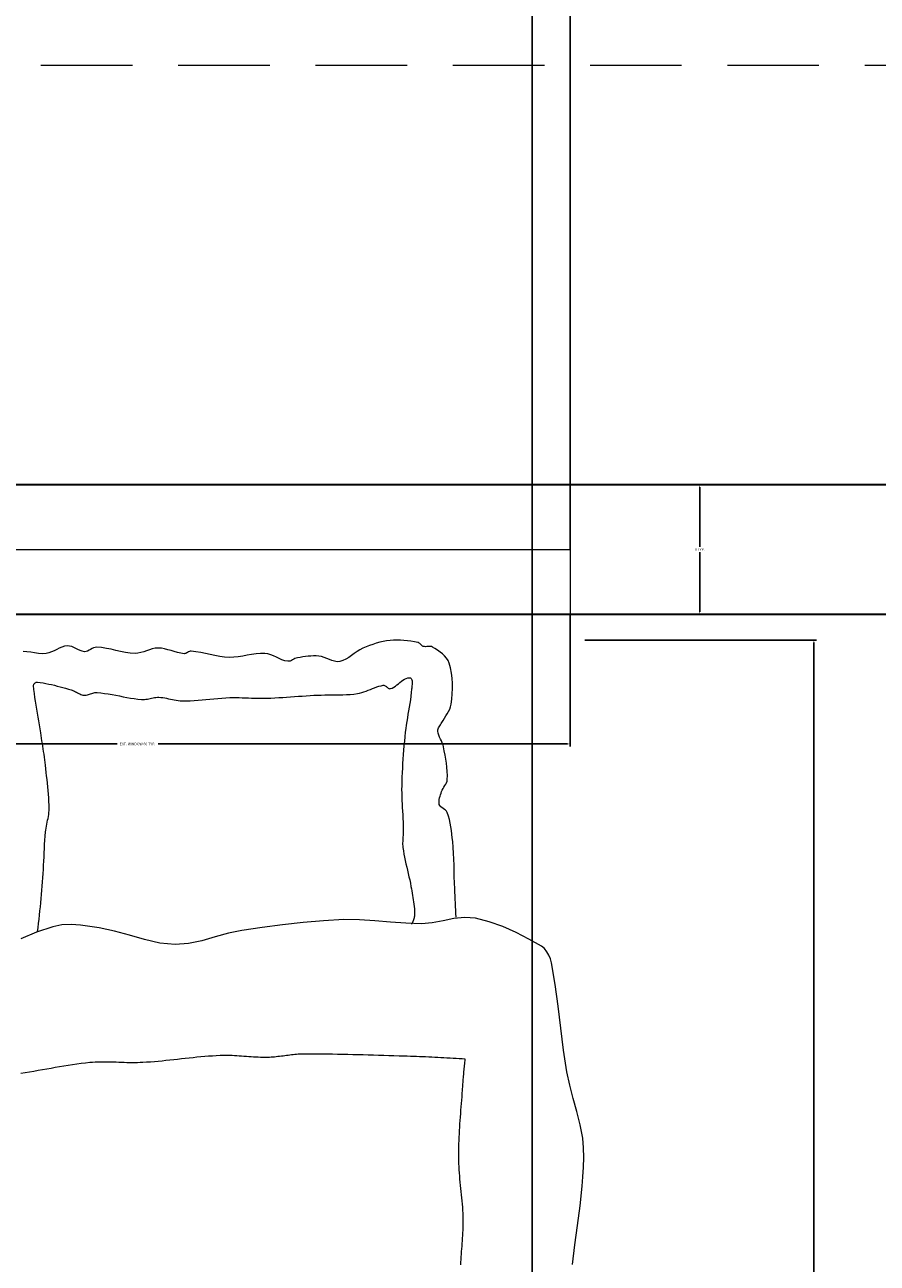
# Model space of a CAD drawing. Units: inches. Extents: x 1770 to 2988, y 1161 to 3221.
# Tile 18 of 44: x 2229 to 2289, y 2323 to 2409. Entities that reach past the tile are written whole.
import ezdxf

# ---------------------------------------------------------------- set-up
doc = ezdxf.new("R2010")
doc.units = ezdxf.units.IN
doc.linetypes.add('DASHED2', pattern=[9.525, 6.35, -3.175])
for name, color, linetype, lineweight in [('A-ANNO-DIMS', 2, 'Continuous', 18), ('A-FURN', 8, 'Continuous', 13), ('A-GLAZ', 4, 'Continuous', 18), ('A-ROOF-OVHD', 7, 'DASHED2', 18), ('A-WALL', 7, 'Continuous', 35)]:
    doc.layers.add(name, color=color, linetype=linetype, lineweight=lineweight)
doc.styles.get("Standard").update_dxf_attribs({"font": 'arial.ttf'})
doc.dimstyles.get("Standard").update_dxf_attribs({"dimtxt": 0.18, "dimasz": 0.18, "dimexe": 0.18, "dimexo": 0.0625, "dimgap": 0.09, "dimtad": 0, "dimtih": 1, "dimtoh": 1, "dimdec": 4, "dimzin": 0, "dimdsep": 46, "dimtxsty": 'Standard', "dimcen": 0.09, "dimadec": 0, "dimazin": 0, "dimtfac": 1, "dimtdec": 4, "dimtofl": 0, "dimtmove": 0, "dimatfit": 3, "dimfxl": 1, "dimtolj": 1, "dimtzin": 0, "dimarcsym": 0})

# ---------------------------------------------------------------- blocks, each defined once
blk = doc.blocks.new('BED-DOUBLE-PLAN')
for p, q in [((38.413, 105.766), (38.234, 105.676)), ((38.593, 105.854), (38.413, 105.766)), ((38.774, 105.931), (38.593, 105.854)), ((38.959, 105.987), (38.774, 105.931)), ((39.151, 106.014), (38.959, 105.987)), ((39.305, 106.003), (39.151, 106.014)), ((39.454, 105.962), (39.305, 106.003)), ((39.599, 105.9), (39.454, 105.962)), ((39.744, 105.827), (39.599, 105.9)), ((39.888, 105.751), (39.744, 105.827)), ((40.034, 105.684), (39.888, 105.751)), ((40.766, 105.763), (40.662, 105.704)), ((40.87, 105.822), (40.766, 105.763)), ((40.976, 105.874), (40.87, 105.822)), ((41.084, 105.909), (40.976, 105.874)), ((41.195, 105.919), (41.084, 105.909)), ((41.529, 105.893), (41.195, 105.919)), ((41.861, 105.841), (41.529, 105.893)), ((42.191, 105.773), (41.861, 105.841)), ((42.521, 105.698), (42.191, 105.773)), ((45.042, 105.801), (44.844, 105.741)), ((45.243, 105.843), (45.042, 105.801)), ((45.446, 105.858), (45.243, 105.843)), ((45.675, 105.843), (45.446, 105.858)), ((45.901, 105.804), (45.675, 105.843)), ((46.126, 105.748), (45.901, 105.804)), ((46.349, 105.683), (46.126, 105.748)), ((59.45, 105.749), (59.252, 105.623)), ((59.658, 105.853), (59.45, 105.749)), ((59.885, 105.946), (59.658, 105.853)), ((60.115, 106.035), (59.885, 105.946)), ((60.348, 106.118), (60.115, 106.035)), ((60.582, 106.193), (60.348, 106.118)), ((60.819, 106.26), (60.582, 106.193)), ((61.059, 106.316), (60.819, 106.26)), ((61.3, 106.362), (61.059, 106.316)), ((61.543, 106.394), (61.3, 106.362)), ((61.783, 106.412), (61.543, 106.394)), ((62.023, 106.417), (61.783, 106.412)), ((62.265, 106.41), (62.023, 106.417)), ((62.506, 106.393), (62.265, 106.41)), ((62.747, 106.368), (62.506, 106.393)), ((62.987, 106.335), (62.747, 106.368)), ((63.226, 106.297), (62.987, 106.335)), ((63.464, 106.255), (63.226, 106.297)), ((63.519, 106.237), (63.464, 106.255)), ((63.567, 106.207), (63.519, 106.237)), ((63.612, 106.167), (63.567, 106.207)), ((63.655, 106.123), (63.612, 106.167)), ((63.698, 106.078), (63.655, 106.123)), ((63.742, 106.036), (63.698, 106.078)), ((63.79, 106), (63.742, 106.036)), ((63.842, 105.976), (63.79, 106)), ((63.921, 105.96), (63.842, 105.976)), ((64.003, 105.957), (63.921, 105.96)), ((64.087, 105.963), (64.003, 105.957)), ((64.171, 105.972), (64.087, 105.963)), ((64.255, 105.978), (64.171, 105.972)), ((64.335, 105.976), (64.255, 105.978)), ((64.412, 105.962), (64.335, 105.976)), ((64.483, 105.93), (64.412, 105.962)), ((64.655, 105.82), (64.483, 105.93)), ((64.831, 105.707), (64.655, 105.82)), ((36.348, 105.604), (36.086, 105.618)), ((36.614, 105.569), (36.348, 105.604)), ((36.882, 105.525), (36.614, 105.569)), ((37.15, 105.487), (36.882, 105.525)), ((37.417, 105.469), (37.15, 105.487)), ((37.679, 105.483), (37.417, 105.469)), ((37.869, 105.525), (37.679, 105.483)), ((38.054, 105.593), (37.869, 105.525)), ((38.234, 105.676), (38.054, 105.593)), ((40.183, 105.634), (40.034, 105.684)), ((40.337, 105.61), (40.183, 105.634)), ((40.448, 105.619), (40.337, 105.61)), ((40.556, 105.654), (40.448, 105.619)), ((40.662, 105.704), (40.556, 105.654)), ((42.85, 105.623), (42.521, 105.698)), ((43.18, 105.557), (42.85, 105.623)), ((43.512, 105.51), (43.18, 105.557)), ((43.846, 105.489), (43.512, 105.51)), ((44.05, 105.503), (43.846, 105.489)), ((44.25, 105.544), (44.05, 105.503)), ((44.449, 105.603), (44.25, 105.544)), ((44.646, 105.672), (44.449, 105.603)), ((44.844, 105.741), (44.646, 105.672)), ((46.572, 105.616), (46.349, 105.683)), ((46.796, 105.553), (46.572, 105.616)), ((47.022, 105.502), (46.796, 105.553)), ((47.25, 105.469), (47.022, 105.502)), ((47.314, 105.472), (47.25, 105.469)), ((47.375, 105.492), (47.314, 105.472)), ((47.436, 105.521), (47.375, 105.492)), ((47.495, 105.556), (47.436, 105.521)), ((47.555, 105.592), (47.495, 105.556)), ((47.615, 105.622), (47.555, 105.592)), ((47.677, 105.641), (47.615, 105.622)), ((47.741, 105.646), (47.677, 105.641)), ((48.074, 105.608), (47.741, 105.646)), ((48.406, 105.552), (48.074, 105.608)), ((48.736, 105.485), (48.406, 105.552)), ((49.065, 105.414), (48.736, 105.485)), ((49.395, 105.345), (49.065, 105.414)), ((49.725, 105.284), (49.395, 105.345)), ((50.057, 105.239), (49.725, 105.284)), ((50.391, 105.215), (50.057, 105.239)), ((50.701, 105.221), (50.391, 105.215)), ((51.01, 105.253), (50.701, 105.221)), ((51.318, 105.302), (51.01, 105.253)), ((51.626, 105.359), (51.318, 105.302)), ((51.934, 105.415), (51.626, 105.359)), ((52.242, 105.46), (51.934, 105.415)), ((52.551, 105.485), (52.242, 105.46)), ((52.86, 105.482), (52.551, 105.485)), ((53.065, 105.451), (52.86, 105.482)), ((53.264, 105.392), (53.065, 105.451)), ((53.459, 105.314), (53.264, 105.392)), ((53.652, 105.225), (53.459, 105.314)), ((53.845, 105.135), (53.652, 105.225)), ((54.039, 105.052), (53.845, 105.135)), ((54.237, 104.985), (54.039, 105.052)), ((54.441, 104.943), (54.237, 104.985)), ((54.528, 104.942), (54.441, 104.943)), ((54.613, 104.962), (54.528, 104.942)), ((54.696, 104.995), (54.613, 104.962)), ((54.779, 105.038), (54.696, 104.995)), ((54.861, 105.083), (54.779, 105.038)), ((54.944, 105.127), (54.861, 105.083)), ((55.029, 105.163), (54.944, 105.127)), ((55.116, 105.186), (55.029, 105.163)), ((55.3, 105.216), (55.116, 105.186)), ((55.484, 105.245), (55.3, 105.216)), ((55.669, 105.271), (55.484, 105.245)), ((55.855, 105.292), (55.669, 105.271)), ((56.041, 105.308), (55.855, 105.292)), ((56.227, 105.316), (56.041, 105.308)), ((56.413, 105.315), (56.227, 105.316)), ((56.598, 105.304), (56.413, 105.315)), ((56.783, 105.272), (56.598, 105.304)), ((56.966, 105.215), (56.783, 105.272)), ((57.147, 105.142), (56.966, 105.215)), ((57.327, 105.066), (57.147, 105.142)), ((57.506, 104.996), (57.327, 105.066)), ((57.686, 104.943), (57.506, 104.996)), ((57.868, 104.916), (57.686, 104.943)), ((58.051, 104.927), (57.868, 104.916)), ((58.271, 104.989), (58.051, 104.927)), ((58.479, 105.084), (58.271, 104.989)), ((58.677, 105.205), (58.479, 105.084)), ((58.869, 105.341), (58.677, 105.205)), ((59.06, 105.484), (58.869, 105.341)), ((59.252, 105.623), (59.06, 105.484)), ((65.005, 105.587), (64.831, 105.707)), ((65.17, 105.459), (65.005, 105.587)), ((65.323, 105.321), (65.17, 105.459)), ((65.456, 105.17), (65.323, 105.321)), ((65.565, 105.005), (65.456, 105.17)), ((65.644, 104.823), (65.565, 105.005)), ((65.74, 104.478), (65.644, 104.823)), ((65.806, 104.126), (65.74, 104.478)), ((65.847, 103.768), (65.806, 104.126)), ((36.815, 103.265), (36.816, 103.295)), ((36.837, 102.989), (36.815, 103.265)), ((36.816, 103.295), (36.824, 103.324)), ((36.824, 103.324), (36.836, 103.353)), ((36.836, 103.353), (36.854, 103.381)), ((36.854, 103.381), (36.875, 103.407)), ((36.875, 103.407), (36.9, 103.431)), ((36.9, 103.431), (36.927, 103.452)), ((36.927, 103.452), (36.956, 103.47)), ((36.956, 103.47), (36.986, 103.485)), ((36.986, 103.485), (37.017, 103.494)), ((37.017, 103.494), (37.048, 103.499)), ((37.048, 103.499), (37.077, 103.499)), ((37.077, 103.499), (37.276, 103.472)), ((37.276, 103.472), (37.474, 103.441)), ((37.474, 103.441), (37.671, 103.405)), ((37.671, 103.405), (37.868, 103.365)), ((37.868, 103.365), (38.063, 103.321)), ((38.063, 103.321), (38.259, 103.274)), ((38.259, 103.274), (38.453, 103.225)), ((38.453, 103.225), (38.648, 103.173)), ((38.648, 103.173), (38.841, 103.121)), ((60.615, 103.161), (60.765, 103.209)), ((60.765, 103.209), (60.917, 103.249)), ((60.917, 103.249), (61.072, 103.279)), ((61.072, 103.279), (61.117, 103.279)), ((61.117, 103.279), (61.16, 103.267)), ((61.16, 103.267), (61.202, 103.246)), ((61.202, 103.246), (61.243, 103.218)), ((61.243, 103.218), (61.284, 103.186)), ((61.284, 103.186), (61.324, 103.152)), ((61.805, 103.148), (61.914, 103.221)), ((61.914, 103.221), (62.02, 103.302)), ((62.02, 103.302), (62.123, 103.389)), ((62.123, 103.389), (62.226, 103.476)), ((62.226, 103.476), (62.33, 103.56)), ((62.33, 103.56), (62.435, 103.637)), ((62.435, 103.637), (62.543, 103.703)), ((62.543, 103.703), (62.655, 103.754)), ((62.655, 103.754), (62.772, 103.787)), ((62.772, 103.787), (62.895, 103.797)), ((62.895, 103.797), (62.954, 103.786)), ((62.954, 103.786), (62.999, 103.756)), ((62.999, 103.756), (63.032, 103.711)), ((63.032, 103.711), (63.054, 103.651)), ((63.053, 103.166), (63.044, 103.088)), ((63.061, 103.249), (63.053, 103.166)), ((63.054, 103.651), (63.067, 103.582)), ((63.069, 103.335), (63.061, 103.249)), ((63.067, 103.582), (63.073, 103.504)), ((63.073, 103.421), (63.069, 103.335)), ((63.073, 103.504), (63.073, 103.421)), ((65.866, 103.406), (65.847, 103.768)), ((65.864, 103.043), (65.866, 103.406)), ((36.865, 102.714), (36.837, 102.989)), ((36.9, 102.439), (36.865, 102.714)), ((36.939, 102.165), (36.9, 102.439)), ((38.841, 103.121), (39.035, 103.067)), ((39.035, 103.067), (39.228, 103.012)), ((39.228, 103.012), (39.421, 102.958)), ((39.421, 102.958), (39.498, 102.933)), ((39.498, 102.933), (39.573, 102.902)), ((39.573, 102.902), (39.647, 102.867)), ((39.647, 102.867), (39.721, 102.83)), ((39.721, 102.83), (39.793, 102.791)), ((39.793, 102.791), (39.866, 102.752)), ((39.866, 102.752), (39.938, 102.714)), ((39.938, 102.714), (40.011, 102.679)), ((40.011, 102.679), (40.086, 102.647)), ((40.086, 102.647), (40.161, 102.62)), ((40.161, 102.62), (40.238, 102.6)), ((40.238, 102.6), (40.317, 102.588)), ((40.317, 102.588), (40.394, 102.585)), ((40.394, 102.585), (40.469, 102.592)), ((40.469, 102.592), (40.544, 102.607)), ((40.544, 102.607), (40.619, 102.627)), ((40.619, 102.627), (40.694, 102.651)), ((40.694, 102.651), (40.769, 102.678)), ((40.769, 102.678), (40.843, 102.704)), ((40.843, 102.704), (40.918, 102.729)), ((40.918, 102.729), (40.993, 102.75)), ((40.993, 102.75), (41.068, 102.766)), ((41.068, 102.766), (41.144, 102.775)), ((41.144, 102.775), (41.22, 102.775)), ((41.22, 102.775), (41.479, 102.75)), ((41.479, 102.75), (41.737, 102.718)), ((41.737, 102.718), (41.994, 102.678)), ((41.994, 102.678), (42.251, 102.633)), ((42.251, 102.633), (42.507, 102.585)), ((42.507, 102.585), (42.763, 102.535)), ((42.763, 102.535), (43.019, 102.485)), ((43.019, 102.485), (43.275, 102.436)), ((43.275, 102.436), (43.532, 102.391)), ((43.532, 102.391), (43.789, 102.351)), ((43.789, 102.351), (44.047, 102.317)), ((44.047, 102.317), (44.306, 102.293)), ((44.505, 102.294), (44.604, 102.306)), ((44.604, 102.306), (44.703, 102.322)), ((44.703, 102.322), (44.802, 102.341)), ((44.802, 102.341), (44.902, 102.363)), ((44.902, 102.363), (45.001, 102.385)), ((45.001, 102.385), (45.1, 102.405)), ((45.1, 102.405), (45.199, 102.423)), ((45.199, 102.423), (45.299, 102.437)), ((45.299, 102.437), (45.398, 102.445)), ((45.398, 102.445), (45.498, 102.446)), ((45.498, 102.446), (45.634, 102.437)), ((45.634, 102.437), (45.769, 102.421)), ((45.769, 102.421), (45.904, 102.399)), ((45.904, 102.399), (46.038, 102.373)), ((46.038, 102.373), (46.172, 102.345)), ((46.172, 102.345), (46.306, 102.315)), ((46.306, 102.315), (46.439, 102.285)), ((48.771, 102.294), (49.047, 102.32)), ((49.047, 102.32), (49.323, 102.346)), ((49.323, 102.346), (49.599, 102.371)), ((49.599, 102.371), (49.876, 102.392)), ((49.876, 102.392), (50.152, 102.409)), ((50.152, 102.409), (50.429, 102.421)), ((50.429, 102.421), (50.643, 102.426)), ((50.643, 102.426), (50.858, 102.426)), ((50.858, 102.426), (51.073, 102.423)), ((51.073, 102.423), (51.288, 102.417)), ((51.288, 102.417), (51.503, 102.41)), ((51.503, 102.41), (51.718, 102.402)), ((51.718, 102.402), (51.933, 102.394)), ((51.933, 102.394), (52.148, 102.387)), ((52.148, 102.387), (52.363, 102.381)), ((52.363, 102.381), (52.578, 102.377)), ((52.578, 102.377), (52.793, 102.377)), ((52.793, 102.377), (53.008, 102.381)), ((53.008, 102.381), (53.279, 102.39)), ((53.279, 102.39), (53.551, 102.403)), ((53.551, 102.403), (53.822, 102.418)), ((53.822, 102.418), (54.093, 102.435)), ((54.093, 102.435), (54.364, 102.453)), ((54.364, 102.453), (54.635, 102.473)), ((54.635, 102.473), (54.906, 102.493)), ((54.906, 102.493), (55.177, 102.513)), ((55.177, 102.513), (55.448, 102.533)), ((55.448, 102.533), (55.719, 102.552)), ((55.719, 102.552), (55.991, 102.569)), ((55.991, 102.569), (56.262, 102.584)), ((56.262, 102.584), (56.513, 102.594)), ((56.513, 102.594), (56.764, 102.6)), ((56.764, 102.6), (57.015, 102.603)), ((57.015, 102.603), (57.267, 102.604)), ((57.267, 102.604), (57.518, 102.605)), ((57.518, 102.605), (57.77, 102.606)), ((57.77, 102.606), (58.021, 102.61)), ((58.021, 102.61), (58.272, 102.616)), ((58.272, 102.616), (58.522, 102.627)), ((58.522, 102.627), (58.773, 102.644)), ((58.773, 102.644), (59.022, 102.667)), ((59.022, 102.667), (59.271, 102.698)), ((59.271, 102.698), (59.425, 102.727)), ((59.425, 102.727), (59.578, 102.766)), ((59.578, 102.766), (59.728, 102.814)), ((59.728, 102.814), (59.876, 102.868)), ((59.876, 102.868), (60.024, 102.927)), ((60.024, 102.927), (60.171, 102.987)), ((60.171, 102.987), (60.319, 103.048)), ((60.319, 103.048), (60.466, 103.107)), ((60.466, 103.107), (60.615, 103.161)), ((61.324, 103.152), (61.364, 103.119)), ((61.364, 103.119), (61.404, 103.088)), ((61.404, 103.088), (61.445, 103.062)), ((61.445, 103.062), (61.487, 103.045)), ((61.487, 103.045), (61.529, 103.038)), ((61.529, 103.038), (61.573, 103.043)), ((61.573, 103.043), (61.691, 103.087)), ((61.691, 103.087), (61.805, 103.148)), ((62.984, 102.514), (62.949, 102.264)), ((63.014, 102.765), (62.984, 102.514)), ((63.038, 103.017), (63.014, 102.765)), ((63.044, 103.088), (63.038, 103.017)), ((65.776, 101.96), (65.816, 102.318)), ((65.816, 102.318), (65.847, 102.679)), ((65.847, 102.679), (65.864, 103.043)), ((36.982, 101.891), (36.939, 102.165)), ((37.028, 101.618), (36.982, 101.891)), ((37.075, 101.344), (37.028, 101.618)), ((44.306, 102.293), (44.405, 102.29)), ((44.405, 102.29), (44.505, 102.294)), ((46.439, 102.285), (46.573, 102.258)), ((46.573, 102.258), (46.708, 102.234)), ((46.708, 102.234), (46.842, 102.214)), ((46.842, 102.214), (46.977, 102.201)), ((46.977, 102.201), (47.113, 102.196)), ((47.113, 102.196), (47.39, 102.199)), ((47.39, 102.199), (47.666, 102.208)), ((47.666, 102.208), (47.943, 102.224)), ((47.943, 102.224), (48.219, 102.244)), ((48.219, 102.244), (48.495, 102.268)), ((48.495, 102.268), (48.771, 102.294)), ((62.825, 101.515), (62.781, 101.266)), ((62.869, 101.765), (62.825, 101.515)), ((62.91, 102.014), (62.869, 101.765)), ((62.949, 102.264), (62.91, 102.014)), ((65.508, 101.305), (65.6, 101.461)), ((65.6, 101.461), (65.679, 101.621)), ((65.679, 101.621), (65.74, 101.786)), ((65.74, 101.786), (65.776, 101.96)), ((37.124, 101.071), (37.075, 101.344)), ((37.173, 100.798), (37.124, 101.071)), ((37.22, 100.525), (37.173, 100.798)), ((62.697, 100.767), (62.658, 100.517)), ((62.738, 101.017), (62.697, 100.767)), ((62.781, 101.266), (62.738, 101.017)), ((65.041, 100.543), (65.086, 100.614)), ((65.086, 100.614), (65.126, 100.685)), ((65.126, 100.685), (65.213, 100.843)), ((65.213, 100.843), (65.309, 100.998)), ((65.309, 100.998), (65.409, 101.151)), ((65.409, 101.151), (65.508, 101.305)), ((37.265, 100.251), (37.22, 100.525)), ((37.308, 99.977), (37.265, 100.251)), ((37.335, 99.791), (37.308, 99.977)), ((37.364, 99.604), (37.335, 99.791)), ((62.595, 100.015), (62.564, 99.705)), ((62.624, 100.266), (62.595, 100.015)), ((62.658, 100.517), (62.624, 100.266)), ((64.852, 100.101), (64.855, 100.18)), ((64.874, 99.957), (64.852, 100.101)), ((64.855, 100.18), (64.874, 100.256)), ((64.874, 100.256), (64.906, 100.33)), ((64.915, 99.818), (64.874, 99.957)), ((64.906, 100.33), (64.947, 100.402)), ((64.97, 99.682), (64.915, 99.818)), ((64.947, 100.402), (64.993, 100.473)), ((64.993, 100.473), (65.041, 100.543)), ((37.393, 99.418), (37.364, 99.604)), ((37.422, 99.231), (37.393, 99.418)), ((37.451, 99.045), (37.422, 99.231)), ((37.479, 98.858), (37.451, 99.045)), ((62.506, 99.085), (62.479, 98.774)), ((62.534, 99.395), (62.506, 99.085)), ((62.564, 99.705), (62.534, 99.395)), ((65.033, 99.547), (64.97, 99.682)), ((65.098, 99.412), (65.033, 99.547)), ((65.16, 99.277), (65.098, 99.412)), ((65.212, 99.139), (65.16, 99.277)), ((65.25, 98.997), (65.212, 99.139)), ((65.304, 98.717), (65.25, 98.997)), ((37.507, 98.672), (37.479, 98.858)), ((37.534, 98.485), (37.507, 98.672)), ((37.56, 98.298), (37.534, 98.485)), ((37.585, 98.111), (37.56, 98.298)), ((37.609, 97.924), (37.585, 98.111)), ((62.432, 98.153), (62.411, 97.842)), ((62.455, 98.464), (62.432, 98.153)), ((62.479, 98.774), (62.455, 98.464)), ((65.357, 98.436), (65.304, 98.717)), ((65.405, 98.154), (65.357, 98.436)), ((65.447, 97.871), (65.405, 98.154)), ((37.63, 97.737), (37.609, 97.924)), ((37.659, 97.485), (37.63, 97.737)), ((37.688, 97.233), (37.659, 97.485)), ((37.717, 96.982), (37.688, 97.233)), ((62.377, 97.22), (62.364, 96.909)), ((62.393, 97.531), (62.377, 97.22)), ((62.411, 97.842), (62.393, 97.531)), ((65.481, 97.587), (65.447, 97.871)), ((65.504, 97.303), (65.481, 97.587)), ((65.515, 97.019), (65.504, 97.303)), ((37.746, 96.73), (37.717, 96.982)), ((37.774, 96.478), (37.746, 96.73)), ((37.801, 96.226), (37.774, 96.478)), ((62.346, 96.286), (62.343, 96.035)), ((62.353, 96.597), (62.346, 96.286)), ((62.364, 96.909), (62.353, 96.597)), ((65.281, 96.212), (65.346, 96.312)), ((65.346, 96.312), (65.406, 96.413)), ((65.406, 96.413), (65.458, 96.516)), ((65.458, 96.516), (65.494, 96.622)), ((65.494, 96.622), (65.511, 96.734)), ((65.511, 96.734), (65.515, 97.019)), ((37.825, 95.974), (37.801, 96.226)), ((37.846, 95.722), (37.825, 95.974)), ((37.864, 95.469), (37.846, 95.722)), ((37.877, 95.217), (37.864, 95.469)), ((62.343, 96.035), (62.346, 95.785)), ((62.346, 95.785), (62.352, 95.534)), ((62.352, 95.534), (62.362, 95.283)), ((64.948, 95.343), (64.973, 95.456)), ((64.973, 95.456), (65.006, 95.569)), ((65.006, 95.569), (65.043, 95.68)), ((65.043, 95.68), (65.082, 95.791)), ((65.082, 95.791), (65.119, 95.9)), ((65.119, 95.9), (65.162, 96.007)), ((65.162, 96.007), (65.218, 96.11)), ((65.218, 96.11), (65.281, 96.212)), ((37.875, 94.44), (37.886, 94.575)), ((37.886, 94.964), (37.877, 95.217)), ((37.89, 94.711), (37.886, 94.964)), ((37.886, 94.575), (37.89, 94.711)), ((62.362, 95.283), (62.374, 95.032)), ((62.374, 95.032), (62.388, 94.782)), ((62.388, 94.782), (62.403, 94.531)), ((64.935, 95.231), (64.948, 95.343)), ((64.936, 95.119), (64.935, 95.231)), ((64.955, 95.009), (64.936, 95.119)), ((64.994, 94.922), (64.955, 95.009)), ((65.057, 94.848), (64.994, 94.922)), ((65.135, 94.784), (65.057, 94.848)), ((65.222, 94.724), (65.135, 94.784)), ((65.31, 94.665), (65.222, 94.724)), ((65.391, 94.601), (65.31, 94.665)), ((65.459, 94.53), (65.391, 94.601)), ((37.727, 93.635), (37.755, 93.769)), ((37.755, 93.769), (37.783, 93.903)), ((37.783, 93.903), (37.811, 94.037)), ((37.811, 94.037), (37.836, 94.171)), ((37.836, 94.171), (37.858, 94.305)), ((37.858, 94.305), (37.875, 94.44)), ((62.403, 94.531), (62.417, 94.28)), ((62.417, 94.28), (62.431, 94.03)), ((62.431, 94.03), (62.443, 93.779)), ((62.443, 93.779), (62.453, 93.528)), ((65.505, 94.445), (65.459, 94.53)), ((65.585, 94.202), (65.505, 94.445)), ((65.653, 93.955), (65.585, 94.202)), ((65.709, 93.705), (65.653, 93.955)), ((37.616, 92.807), (37.64, 93.096)), ((37.64, 93.096), (37.655, 93.231)), ((37.655, 93.231), (37.676, 93.366)), ((37.676, 93.366), (37.7, 93.501)), ((37.7, 93.501), (37.727, 93.635)), ((62.443, 92.857), (62.435, 92.752)), ((62.451, 92.962), (62.443, 92.857)), ((62.457, 93.067), (62.451, 92.962)), ((62.453, 93.528), (62.46, 93.277)), ((62.46, 93.172), (62.457, 93.067)), ((62.46, 93.277), (62.46, 93.172)), ((65.756, 93.453), (65.709, 93.705)), ((65.796, 93.198), (65.756, 93.453)), ((65.829, 92.943), (65.796, 93.198)), ((65.858, 92.688), (65.829, 92.943)), ((37.562, 91.94), (37.578, 92.229)), ((37.578, 92.229), (37.596, 92.518)), ((37.596, 92.518), (37.616, 92.807)), ((62.414, 92.436), (62.411, 92.332)), ((62.411, 92.332), (62.412, 92.227)), ((62.412, 92.227), (62.418, 92.123)), ((62.419, 92.541), (62.414, 92.436)), ((62.418, 92.123), (62.429, 92.018)), ((62.427, 92.647), (62.419, 92.541)), ((62.435, 92.752), (62.427, 92.647)), ((62.429, 92.018), (62.462, 91.79)), ((65.884, 92.433), (65.858, 92.688)), ((65.919, 92.024), (65.884, 92.433)), ((65.945, 91.615), (65.919, 92.024)), ((37.521, 91.072), (37.534, 91.361)), ((37.534, 91.361), (37.548, 91.651)), ((37.548, 91.651), (37.562, 91.94)), ((62.462, 91.79), (62.502, 91.563)), ((62.502, 91.563), (62.545, 91.337)), ((62.545, 91.337), (62.593, 91.112)), ((65.963, 91.206), (65.945, 91.615)), ((65.977, 90.796), (65.963, 91.206)), ((37.476, 90.204), (37.492, 90.493)), ((37.492, 90.493), (37.507, 90.782)), ((37.507, 90.782), (37.521, 91.072)), ((62.593, 91.112), (62.643, 90.886)), ((62.643, 90.886), (62.694, 90.661)), ((62.694, 90.661), (62.747, 90.437)), ((62.747, 90.437), (62.8, 90.212)), ((65.988, 90.386), (65.977, 90.796)), ((65.998, 89.976), (65.988, 90.386)), ((37.412, 89.337), (37.436, 89.626)), ((37.436, 89.626), (37.457, 89.915)), ((37.457, 89.915), (37.476, 90.204)), ((62.8, 90.212), (62.851, 89.987)), ((62.851, 89.987), (62.901, 89.762)), ((62.901, 89.762), (62.947, 89.536)), ((62.947, 89.536), (62.99, 89.309)), ((66.01, 89.566), (65.998, 89.976)), ((66.026, 89.156), (66.01, 89.566)), ((37.336, 88.473), (37.362, 88.761)), ((37.362, 88.761), (37.388, 89.049)), ((37.388, 89.049), (37.412, 89.337)), ((62.99, 89.309), (63.018, 89.156)), ((63.018, 89.156), (63.046, 89.003)), ((63.046, 89.003), (63.074, 88.849)), ((63.074, 88.849), (63.101, 88.696)), ((63.101, 88.696), (63.128, 88.542)), ((66.037, 88.909), (66.026, 89.156)), ((66.048, 88.662), (66.037, 88.909)), ((66.059, 88.415), (66.048, 88.662)), ((37.25, 87.609), (37.279, 87.897)), ((37.279, 87.897), (37.308, 88.185)), ((37.308, 88.185), (37.336, 88.473)), ((63.128, 88.542), (63.153, 88.388)), ((63.153, 88.388), (63.175, 88.234)), ((63.175, 88.234), (63.196, 88.079)), ((63.196, 88.079), (63.213, 87.925)), ((63.213, 87.925), (63.227, 87.77)), ((63.227, 87.77), (63.236, 87.614)), ((66.07, 88.167), (66.059, 88.415)), ((66.081, 87.92), (66.07, 88.167)), ((66.092, 87.673), (66.081, 87.92)), ((37.155, 86.747), (37.188, 87.034)), ((37.188, 87.034), (37.219, 87.322)), ((37.219, 87.322), (37.25, 87.609)), ((56.922, 86.931), (55.503, 86.807)), ((58.343, 87.01), (56.922, 86.931)), ((59.417, 87.004), (58.343, 87.01)), ((60.491, 86.934), (59.417, 87.004)), ((61.564, 86.838), (60.491, 86.934)), ((62.638, 86.756), (61.564, 86.838)), ((63.124, 86.869), (63.097, 86.808)), ((63.149, 86.932), (63.124, 86.869)), ((63.171, 86.996), (63.149, 86.932)), ((63.19, 87.06), (63.171, 86.996)), ((63.207, 87.126), (63.19, 87.06)), ((63.22, 87.192), (63.207, 87.126)), ((63.23, 87.259), (63.22, 87.192)), ((63.237, 87.326), (63.23, 87.259)), ((63.236, 87.614), (63.241, 87.459)), ((63.241, 87.392), (63.237, 87.326)), ((63.241, 87.459), (63.241, 87.392)), ((65.218, 86.934), (64.466, 86.795)), ((65.968, 87.079), (65.218, 86.934)), ((66.715, 87.159), (65.968, 87.079)), ((66.104, 87.426), (66.092, 87.673)), ((66.115, 87.178), (66.104, 87.426)), ((67.458, 87.108), (66.715, 87.159)), ((68.424, 86.867), (67.458, 87.108)), ((69.364, 86.53), (68.424, 86.867)), ((37.023, 86.135), (35.936, 85.668)), ((38.141, 86.518), (37.023, 86.135)), ((37.087, 86.172), (37.121, 86.46)), ((37.121, 86.46), (37.155, 86.747)), ((38.769, 86.641), (38.141, 86.518)), ((39.413, 86.663), (38.769, 86.641)), ((40.065, 86.616), (39.413, 86.663)), ((40.717, 86.529), (40.065, 86.616)), ((41.361, 86.431), (40.717, 86.529)), ((42.419, 86.215), (41.361, 86.431)), ((43.465, 85.923), (42.419, 86.215)), ((50.335, 86.067), (49.413, 85.808)), ((51.266, 86.26), (50.335, 86.067)), ((52.675, 86.462), (51.266, 86.26)), ((54.088, 86.648), (52.675, 86.462)), ((55.503, 86.807), (54.088, 86.648)), ((63.713, 86.728), (62.638, 86.756)), ((63.066, 86.748), (63.033, 86.691)), ((63.097, 86.808), (63.066, 86.748)), ((64.466, 86.795), (63.713, 86.728)), ((70.28, 86.118), (69.364, 86.53)), ((71.172, 85.653), (70.28, 86.118)), ((44.51, 85.624), (43.465, 85.923)), ((45.561, 85.387), (44.51, 85.624)), ((46.628, 85.281), (45.561, 85.387)), ((47.567, 85.35), (46.628, 85.281)), ((48.493, 85.547), (47.567, 85.35)), ((49.413, 85.808), (48.493, 85.547)), ((72.043, 85.157), (71.172, 85.653)), ((72.253, 84.994), (72.043, 85.157)), ((72.425, 84.785), (72.253, 84.994)), ((72.561, 84.542), (72.425, 84.785)), ((72.662, 84.282), (72.561, 84.542)), ((72.731, 84.019), (72.662, 84.282)), ((72.993, 82.51), (72.731, 84.019)), ((73.197, 80.991), (72.993, 82.51)), ((73.377, 79.468), (73.197, 80.991)), ((73.567, 77.947), (73.377, 79.468)), ((47.605, 77.397), (47.337, 77.368)), ((47.873, 77.425), (47.605, 77.397)), ((48.142, 77.452), (47.873, 77.425)), ((48.41, 77.477), (48.142, 77.452)), ((48.679, 77.501), (48.41, 77.477)), ((48.948, 77.522), (48.679, 77.501)), ((49.216, 77.541), (48.948, 77.522)), ((49.486, 77.557), (49.216, 77.541)), ((49.755, 77.57), (49.486, 77.557)), ((49.92, 77.575), (49.755, 77.57)), ((50.085, 77.577), (49.92, 77.575)), ((50.25, 77.576), (50.085, 77.577)), ((50.415, 77.573), (50.25, 77.576)), ((50.581, 77.567), (50.415, 77.573)), ((50.746, 77.559), (50.581, 77.567)), ((50.911, 77.55), (50.746, 77.559)), ((51.076, 77.54), (50.911, 77.55)), ((51.241, 77.529), (51.076, 77.54)), ((51.406, 77.517), (51.241, 77.529)), ((51.571, 77.505), (51.406, 77.517)), ((51.737, 77.493), (51.571, 77.505)), ((51.902, 77.482), (51.737, 77.493)), ((52.067, 77.472), (51.902, 77.482)), ((52.232, 77.462), (52.067, 77.472)), ((52.397, 77.455), (52.232, 77.462)), ((52.562, 77.448), (52.397, 77.455)), ((52.728, 77.444), (52.562, 77.448)), ((52.893, 77.443), (52.728, 77.444)), ((53.058, 77.444), (52.893, 77.443)), ((53.176, 77.448), (53.058, 77.444)), ((53.294, 77.454), (53.176, 77.448)), ((53.411, 77.462), (53.294, 77.454)), ((53.528, 77.472), (53.411, 77.462)), ((53.646, 77.484), (53.528, 77.472)), ((53.763, 77.497), (53.646, 77.484)), ((53.88, 77.511), (53.763, 77.497)), ((53.997, 77.526), (53.88, 77.511)), ((54.114, 77.542), (53.997, 77.526)), ((54.231, 77.558), (54.114, 77.542)), ((54.348, 77.574), (54.231, 77.558)), ((54.465, 77.589), (54.348, 77.574)), ((54.582, 77.604), (54.465, 77.589)), ((54.7, 77.618), (54.582, 77.604)), ((54.817, 77.631), (54.7, 77.618)), ((54.934, 77.642), (54.817, 77.631)), ((55.051, 77.651), (54.934, 77.642)), ((55.169, 77.659), (55.051, 77.651)), ((55.286, 77.664), (55.169, 77.659)), ((55.404, 77.666), (55.286, 77.664)), ((55.76, 77.669), (55.404, 77.666)), ((56.116, 77.67), (55.76, 77.669)), ((56.472, 77.669), (56.116, 77.67)), ((56.828, 77.667), (56.472, 77.669)), ((57.184, 77.664), (56.828, 77.667)), ((57.54, 77.66), (57.184, 77.664)), ((57.896, 77.655), (57.54, 77.66)), ((58.252, 77.648), (57.896, 77.655)), ((58.608, 77.641), (58.252, 77.648)), ((58.964, 77.633), (58.608, 77.641)), ((59.32, 77.625), (58.964, 77.633)), ((59.676, 77.615), (59.32, 77.625)), ((60.032, 77.606), (59.676, 77.615)), ((60.388, 77.595), (60.032, 77.606)), ((60.744, 77.585), (60.388, 77.595)), ((61.1, 77.574), (60.744, 77.585)), ((61.456, 77.563), (61.1, 77.574)), ((61.812, 77.552), (61.456, 77.563)), ((62.168, 77.541), (61.812, 77.552)), ((62.524, 77.53), (62.168, 77.541)), ((62.736, 77.524), (62.524, 77.53)), ((62.947, 77.517), (62.736, 77.524)), ((63.159, 77.509), (62.947, 77.517)), ((63.371, 77.502), (63.159, 77.509)), ((63.583, 77.494), (63.371, 77.502)), ((63.795, 77.485), (63.583, 77.494)), ((64.006, 77.476), (63.795, 77.485)), ((64.218, 77.467), (64.006, 77.476)), ((64.43, 77.457), (64.218, 77.467)), ((64.642, 77.447), (64.43, 77.457)), ((64.853, 77.436), (64.642, 77.447)), ((65.065, 77.425), (64.853, 77.436)), ((65.276, 77.414), (65.065, 77.425)), ((65.488, 77.402), (65.276, 77.414)), ((65.7, 77.39), (65.488, 77.402)), ((65.911, 77.378), (65.7, 77.39)), ((66.123, 77.365), (65.911, 77.378)), ((73.802, 76.433), (73.567, 77.947)), ((37.125, 76.526), (36.827, 76.474)), ((37.423, 76.579), (37.125, 76.526)), ((37.721, 76.632), (37.423, 76.579)), ((38.019, 76.686), (37.721, 76.632)), ((38.317, 76.738), (38.019, 76.686)), ((38.615, 76.79), (38.317, 76.738)), ((38.914, 76.84), (38.615, 76.79)), ((39.212, 76.888), (38.914, 76.84)), ((39.511, 76.934), (39.212, 76.888)), ((39.811, 76.976), (39.511, 76.934)), ((40.11, 77.016), (39.811, 76.976)), ((40.411, 77.051), (40.11, 77.016)), ((40.712, 77.082), (40.411, 77.051)), ((40.894, 77.097), (40.712, 77.082)), ((41.077, 77.108), (40.894, 77.097)), ((41.261, 77.116), (41.077, 77.108)), ((41.444, 77.121), (41.261, 77.116)), ((41.627, 77.122), (41.444, 77.121)), ((41.811, 77.122), (41.627, 77.122)), ((41.995, 77.119), (41.811, 77.122)), ((42.178, 77.115), (41.995, 77.119)), ((42.362, 77.11), (42.178, 77.115)), ((42.546, 77.104), (42.362, 77.11)), ((42.73, 77.097), (42.546, 77.104)), ((42.914, 77.091), (42.73, 77.097)), ((43.097, 77.085), (42.914, 77.091)), ((43.281, 77.08), (43.097, 77.085)), ((43.465, 77.076), (43.281, 77.08)), ((43.649, 77.074), (43.465, 77.076)), ((43.833, 77.073), (43.649, 77.074)), ((44.016, 77.076), (43.833, 77.073)), ((44.2, 77.081), (44.016, 77.076)), ((44.383, 77.089), (44.2, 77.081)), ((44.652, 77.105), (44.383, 77.089)), ((44.921, 77.124), (44.652, 77.105)), ((45.19, 77.145), (44.921, 77.124)), ((45.459, 77.169), (45.19, 77.145)), ((45.727, 77.194), (45.459, 77.169)), ((45.996, 77.222), (45.727, 77.194)), ((46.264, 77.25), (45.996, 77.222)), ((46.532, 77.279), (46.264, 77.25)), ((46.8, 77.308), (46.532, 77.279)), ((47.068, 77.338), (46.8, 77.308)), ((47.337, 77.368), (47.068, 77.338)), ((66.334, 77.352), (66.123, 77.365)), ((66.546, 77.338), (66.334, 77.352)), ((66.757, 77.324), (66.546, 77.338)), ((66.667, 76.465), (66.677, 76.573)), ((66.677, 76.573), (66.688, 76.68)), ((66.688, 76.68), (66.699, 76.788)), ((66.699, 76.788), (66.71, 76.895)), ((66.71, 76.895), (66.721, 77.002)), ((66.721, 77.002), (66.733, 77.11)), ((66.733, 77.11), (66.745, 77.217)), ((66.745, 77.217), (66.757, 77.324)), ((36.23, 76.374), (35.931, 76.327)), ((36.528, 76.423), (36.23, 76.374)), ((36.827, 76.474), (36.528, 76.423)), ((66.593, 75.605), (66.601, 75.712)), ((66.601, 75.712), (66.61, 75.82)), ((66.61, 75.82), (66.619, 75.928)), ((66.619, 75.928), (66.628, 76.035)), ((66.628, 76.035), (66.637, 76.143)), ((66.637, 76.143), (66.647, 76.25)), ((66.647, 76.25), (66.657, 76.358)), ((66.657, 76.358), (66.667, 76.465)), ((74.003, 75.51), (73.802, 76.433)), ((66.53, 74.708), (66.546, 74.941)), ((66.546, 74.941), (66.562, 75.174)), ((66.562, 75.174), (66.569, 75.282)), ((66.569, 75.282), (66.577, 75.39)), ((66.577, 75.39), (66.585, 75.497)), ((66.585, 75.497), (66.593, 75.605)), ((74.25, 74.596), (74.003, 75.51)), ((66.459, 73.775), (66.477, 74.008)), ((66.477, 74.008), (66.495, 74.241)), ((66.495, 74.241), (66.512, 74.474)), ((66.512, 74.474), (66.53, 74.708)), ((74.506, 73.685), (74.25, 74.596)), ((66.391, 72.841), (66.407, 73.075)), ((66.407, 73.075), (66.424, 73.308)), ((66.424, 73.308), (66.441, 73.541)), ((66.441, 73.541), (66.459, 73.775)), ((74.736, 72.768), (74.506, 73.685)), ((66.348, 72.141), (66.361, 72.375)), ((66.361, 72.375), (66.376, 72.608)), ((66.376, 72.608), (66.391, 72.841)), ((74.904, 71.84), (74.736, 72.768)), ((66.311, 71.207), (66.318, 71.441)), ((66.318, 71.441), (66.326, 71.674)), ((66.326, 71.674), (66.337, 71.908)), ((66.337, 71.908), (66.348, 72.141)), ((74.965, 71.175), (74.904, 71.84)), ((66.304, 70.74), (66.307, 70.974)), ((66.304, 70.506), (66.304, 70.74)), ((66.308, 70.29), (66.304, 70.506)), ((66.307, 70.974), (66.311, 71.207)), ((74.957, 69.836), (74.978, 70.506)), ((74.978, 70.506), (74.965, 71.175)), ((66.315, 70.073), (66.308, 70.29)), ((66.325, 69.857), (66.315, 70.073)), ((66.338, 69.64), (66.325, 69.857)), ((66.354, 69.424), (66.338, 69.64)), ((74.914, 69.165), (74.957, 69.836)), ((66.372, 69.208), (66.354, 69.424)), ((66.391, 68.992), (66.372, 69.208)), ((66.412, 68.776), (66.391, 68.992)), ((66.434, 68.56), (66.412, 68.776)), ((74.862, 68.497), (74.914, 69.165)), ((66.456, 68.344), (66.434, 68.56)), ((66.478, 68.128), (66.456, 68.344)), ((66.5, 67.912), (66.478, 68.128)), ((74.721, 67.139), (74.862, 68.497)), ((66.521, 67.696), (66.5, 67.912)), ((66.541, 67.48), (66.521, 67.696)), ((66.56, 67.264), (66.541, 67.48)), ((66.577, 67.048), (66.56, 67.264)), ((74.536, 65.785), (74.721, 67.139)), ((66.591, 66.832), (66.577, 67.048)), ((66.603, 66.615), (66.591, 66.832)), ((66.611, 66.399), (66.603, 66.615)), ((66.616, 66.182), (66.611, 66.399)), ((66.597, 65.263), (66.605, 65.446)), ((66.605, 65.446), (66.611, 65.63)), ((66.611, 65.63), (66.616, 65.814)), ((66.617, 65.998), (66.616, 66.182)), ((66.616, 65.814), (66.617, 65.998)), ((74.348, 64.431), (74.536, 65.785)), ((66.536, 64.344), (66.55, 64.528)), ((66.55, 64.528), (66.563, 64.711)), ((66.563, 64.711), (66.576, 64.895)), ((66.576, 64.895), (66.587, 65.079)), ((66.587, 65.079), (66.597, 65.263)), ((66.478, 63.609), (66.492, 63.793)), ((66.492, 63.793), (66.506, 63.976)), ((66.506, 63.976), (66.521, 64.16)), ((66.521, 64.16), (66.536, 64.344)), ((74.196, 63.075), (74.348, 64.431)), ((66.441, 63.058), (66.452, 63.241)), ((66.452, 63.241), (66.465, 63.425)), ((66.465, 63.425), (66.478, 63.609))]:
    blk.add_line(p, q)
blk = doc.blocks.new('WIN-60-EXT')
for p, q in [((0, 9), (0, 0)), ((60, 4.5), (60, 9)), ((60, 9), (60, 0)), ((0, 0), (0, 4.5)), ((0, 4.5), (60, 4.5))]:
    blk.add_line(p, q)
blk = doc.blocks.new('*D30')
at = {"layer": 'A-ANNO-DIMS', "color": 0, "lineweight": -2, "transparency": 16777216}
for p, q in [((2207.278, 2367.64), (2207.278, 2358.522)), ((2267.278, 2367.64), (2267.278, 2358.522)), ((2207.458, 2358.702), (2235.853, 2358.702)), ((2267.098, 2358.702), (2238.702, 2358.702))]:
    blk.add_line(p, q, dxfattribs=at)
at = {"layer": 'A-ANNO-DIMS', "color": 0, "transparency": 16777216}
for points in [[(2207.458, 2358.732), (2207.458, 2358.672), (2207.278, 2358.702)], [(2267.098, 2358.732), (2267.098, 2358.672), (2267.278, 2358.702)]]:
    blk.add_solid(points, dxfattribs=at)
at = {"layer": 'Defpoints', "color": 0, "transparency": 16777216}
for p in [(2207.278, 2367.702), (2267.278, 2367.702), (2267.278, 2358.702)]:
    blk.add_point(p, dxfattribs=at)
at = {"layer": 'A-ANNO-DIMS', "color": 0, "transparency": 16777216, "insert": (2237.278, 2358.702), "char_height": 0.18, "attachment_point": 5}
blk.add_mtext('\\A1;EXT. WINDOW 60 TYP.', dxfattribs=at)
blk = doc.blocks.new('*D31')
at = {"layer": 'A-ANNO-DIMS', "color": 0, "lineweight": -2, "transparency": 16777216}
for p, q in [((2267.34, 2376.702), (2276.458, 2376.702)), ((2276.278, 2376.522), (2276.278, 2372.384)), ((2276.278, 2367.882), (2276.278, 2372.02)), ((2267.34, 2367.702), (2276.458, 2367.702))]:
    blk.add_line(p, q, dxfattribs=at)
at = {"layer": 'A-ANNO-DIMS', "color": 0, "transparency": 16777216}
for points in [[(2276.248, 2376.522), (2276.308, 2376.522), (2276.278, 2376.702)], [(2276.248, 2367.882), (2276.308, 2367.882), (2276.278, 2367.702)]]:
    blk.add_solid(points, dxfattribs=at)
at = {"layer": 'Defpoints', "color": 0, "transparency": 16777216}
for p in [(2267.278, 2376.702), (2276.278, 2376.702), (2267.278, 2367.702)]:
    blk.add_point(p, dxfattribs=at)
at = {"layer": 'A-ANNO-DIMS', "color": 0, "transparency": 16777216, "insert": (2276.278, 2372.202), "char_height": 0.18, "attachment_point": 5}
blk.add_mtext('\\A1;9 TYP.', dxfattribs=at)
blk = doc.blocks.new('*D38')
at = {"layer": 'A-ANNO-DIMS', "color": 0, "lineweight": -2, "transparency": 16777216}
for p, q in [((2268.294, 2365.915), (2284.374, 2365.915)), ((2284.194, 2365.735), (2284.194, 2312.889)), ((2284.194, 2259.678), (2284.194, 2312.525)), ((2268.294, 2259.498), (2284.374, 2259.498))]:
    blk.add_line(p, q, dxfattribs=at)
at = {"layer": 'A-ANNO-DIMS', "color": 0, "transparency": 16777216}
for points in [[(2284.164, 2365.735), (2284.224, 2365.735), (2284.194, 2365.915)], [(2284.164, 2259.678), (2284.224, 2259.678), (2284.194, 2259.498)]]:
    blk.add_solid(points, dxfattribs=at)
at = {"layer": 'Defpoints', "color": 0, "transparency": 16777216}
for p in [(2268.232, 2365.915), (2284.194, 2365.915), (2268.232, 2259.498)]:
    blk.add_point(p, dxfattribs=at)
at = {"layer": 'A-ANNO-DIMS', "color": 0, "transparency": 16777216, "insert": (2284.194, 2312.707), "char_height": 0.18, "attachment_point": 5}
blk.add_mtext('\\A1;BED 106 TYP.', dxfattribs=at)
blk = doc.blocks.new('*D65')
at = {"layer": 'A-ANNO-DIMS', "color": 0, "lineweight": -2, "transparency": 16777216}
for p, q in [((2267.278, 2376.765), (2267.278, 2570.705)), ((2267.458, 2570.525), (2320.239, 2570.525)), ((2373.791, 2570.525), (2321.01, 2570.525)), ((2373.971, 2376.765), (2373.971, 2570.705))]:
    blk.add_line(p, q, dxfattribs=at)
at = {"layer": 'A-ANNO-DIMS', "color": 0, "transparency": 16777216}
for points in [[(2267.458, 2570.555), (2267.458, 2570.495), (2267.278, 2570.525)], [(2373.791, 2570.555), (2373.791, 2570.495), (2373.971, 2570.525)]]:
    blk.add_solid(points, dxfattribs=at)
at = {"layer": 'Defpoints', "color": 0, "transparency": 16777216}
for p in [(2373.971, 2570.525), (2267.278, 2376.702), (2373.971, 2376.702)]:
    blk.add_point(p, dxfattribs=at)
at = {"layer": 'A-ANNO-DIMS', "color": 0, "transparency": 16777216, "insert": (2320.624, 2570.525), "char_height": 0.18, "attachment_point": 5}
blk.add_mtext('\\A1;106.7', dxfattribs=at)
blk = doc.blocks.new('*D73')
at = {"layer": 'A-ANNO-DIMS', "color": 0, "lineweight": -2, "transparency": 16777216}
for p, q in [((2456.133, 2367.702), (1907.104, 2367.702)), ((1907.284, 2367.522), (1907.284, 2319.884)), ((1907.284, 2271.882), (1907.284, 2319.52)), ((2456.133, 2271.702), (1907.104, 2271.702))]:
    blk.add_line(p, q, dxfattribs=at)
at = {"layer": 'A-ANNO-DIMS', "color": 0, "transparency": 16777216}
for points in [[(1907.254, 2367.522), (1907.314, 2367.522), (1907.284, 2367.702)], [(1907.254, 2271.882), (1907.314, 2271.882), (1907.284, 2271.702)]]:
    blk.add_solid(points, dxfattribs=at)
at = {"layer": 'Defpoints', "color": 0, "transparency": 16777216}
for p in [(1907.284, 2367.702), (2456.196, 2367.702), (2456.196, 2271.702)]:
    blk.add_point(p, dxfattribs=at)
at = {"layer": 'A-ANNO-DIMS', "color": 0, "transparency": 16777216, "insert": (1907.284, 2319.702), "char_height": 0.18, "attachment_point": 5}
blk.add_mtext('\\A1;96', dxfattribs=at)
blk = doc.blocks.new('*D80')
at = {"layer": 'A-ANNO-DIMS', "color": 0, "lineweight": -2, "transparency": 16777216}
for p, q in [((2264.657, 1610.265), (2264.657, 2570.705)), ((2264.837, 2570.525), (2314.141, 2570.525)), ((2364.232, 2570.525), (2314.928, 2570.525)), ((2364.412, 1610.265), (2364.412, 2570.705))]:
    blk.add_line(p, q, dxfattribs=at)
at = {"layer": 'A-ANNO-DIMS', "color": 0, "transparency": 16777216}
for points in [[(2264.837, 2570.555), (2264.837, 2570.495), (2264.657, 2570.525)], [(2364.232, 2570.555), (2364.232, 2570.495), (2364.412, 2570.525)]]:
    blk.add_solid(points, dxfattribs=at)
at = {"layer": 'Defpoints', "color": 0, "transparency": 16777216}
for p in [(2364.412, 2570.525), (2264.657, 1610.202), (2364.412, 1610.202)]:
    blk.add_point(p, dxfattribs=at)
at = {"layer": 'A-ANNO-DIMS', "color": 0, "transparency": 16777216, "insert": (2314.534, 2570.525), "char_height": 0.18, "attachment_point": 5}
blk.add_mtext('\\A1;99.76', dxfattribs=at)

msp = doc.modelspace()

# ---------------------------------------------------------------- linework, layer by layer
at = {"layer": 'A-ROOF-OVHD'}
msp.add_line((2656.0216, 2405.7876), (2096.7313, 2405.7876), dxfattribs=at)
at = {"layer": 'A-WALL'}
for p, q in [((2151.696, 2376.7021), (2625.696, 2376.7021)), ((2160.696, 2367.7021), (2328.696, 2367.7021))]:
    msp.add_line(p, q, dxfattribs=at)

# ---------------------------------------------------------------- block references
at = {"layer": 'A-FURN'}
msp.add_blockref('BED-DOUBLE-PLAN', (2193.254, 2259.498), dxfattribs=at)
at = {"layer": 'A-GLAZ'}
msp.add_blockref('WIN-60-EXT', (2207.2778, 2367.702), dxfattribs=at)

# ---------------------------------------------------------------- dimensions: what is measured, and where the dimension line sits
at = {"layer": 'A-ANNO-DIMS'}
for base, p1, p2, override, picture, middle in [((2364.4122, 2570.5247), (2264.6568, 1610.2021), (2364.4122, 1610.2021), {"dimdec": 2, "dimlfac": 1, "dimrnd": 0, "dimzin": 0, "dimdsep": 46, "dimlunit": 2}, '*D80', (2314.5345, 2570.5247)), ((2373.9714, 2570.5247), (2267.2776, 2376.7021), (2373.9714, 2376.7021), {"dimdec": 1, "dimlfac": 1, "dimrnd": 0, "dimzin": 0, "dimdsep": 46, "dimlunit": 2}, '*D65', (2320.6245, 2570.5247))]:
    dim = msp.add_linear_dim(base=base, p1=p1, p2=p2, dimstyle='Standard', override=override, dxfattribs=at)
    dim.commit()
    dim.dimension.update_dxf_attribs({"geometry": picture, "text_midpoint": middle})
for base, p1, p2, text, picture, middle in [((2276.2776, 2376.7021), (2267.2776, 2367.7021), (2267.2776, 2376.7021), '<> TYP.', '*D31', (2276.2776, 2372.2021)), ((2284.1945, 2365.9152), (2268.232, 2259.4983), (2268.232, 2365.9152), 'BED <> TYP.', '*D38', (2284.1945, 2312.7068))]:
    dim = msp.add_linear_dim(base=base, p1=p1, p2=p2, angle=90, text=text, dimstyle='Standard', override={"dimdec": 0, "dimlfac": 1, "dimrnd": 0, "dimzin": 0, "dimdsep": 46, "dimlunit": 2}, dxfattribs=at)
    dim.commit()
    dim.dimension.update_dxf_attribs({"geometry": picture, "text_midpoint": middle})
dim = msp.add_linear_dim(base=(1907.2844, 2367.7021), p1=(2456.196, 2271.7021), p2=(2456.196, 2367.7021), angle=90, dimstyle='Standard', override={"dimdec": 0, "dimlfac": 1, "dimrnd": 0, "dimzin": 0, "dimdsep": 46, "dimlunit": 2}, dxfattribs=at)
dim.commit()
dim.dimension.update_dxf_attribs({"geometry": '*D73', "text_midpoint": (1907.2844, 2319.7021)})
dim = msp.add_linear_dim(base=(2267.2776, 2358.7021), p1=(2207.2776, 2367.7021), p2=(2267.2776, 2367.7021), text='EXT. WINDOW <> TYP.', dimstyle='Standard', override={"dimdec": 0, "dimlfac": 1, "dimrnd": 0, "dimzin": 0, "dimdsep": 46, "dimlunit": 2}, dxfattribs=at)
dim.commit()
dim.dimension.update_dxf_attribs({"geometry": '*D30', "text_midpoint": (2237.2776, 2358.7021)})

doc.saveas('drawing.dxf')
